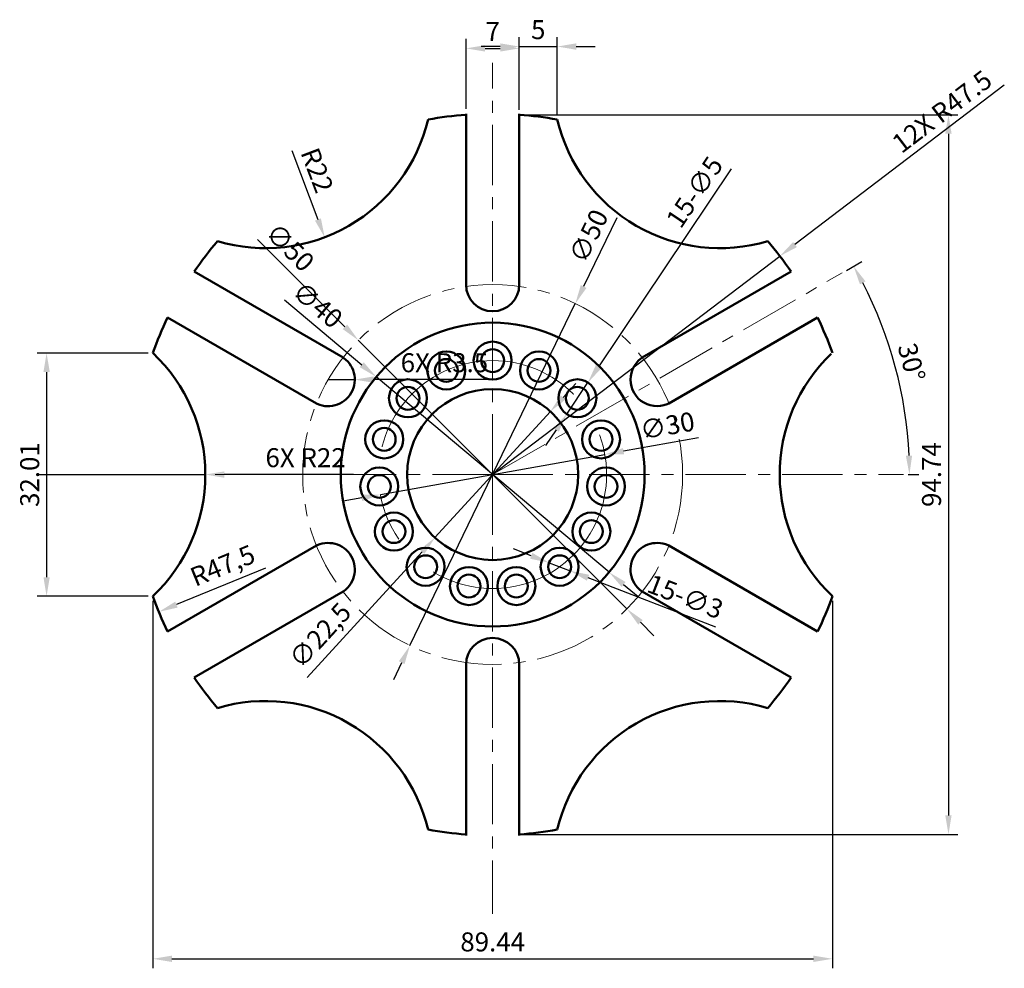
# Model space of a CAD drawing. Units: millimetres. Extents: x 3183 to 3313, y 1440 to 1565.
import ezdxf

# ---------------------------------------------------------------- set-up
doc = ezdxf.new("R2010")
doc.units = ezdxf.units.MM
doc.linetypes.add('CENTER', pattern=[50.8, 31.75, -6.35, 6.35, -6.35])
for name, color, linetype, lineweight in [('M-CNTR', 4, 'CENTER', 18), ('M-DIMS', 2, 'Continuous', 25), ('M-OUTL', 7, 'Continuous', 50)]:
    doc.layers.add(name, color=color, linetype=linetype, lineweight=lineweight)
doc.styles.get("Standard").update_dxf_attribs({"font": 'arial.ttf'})
doc.dimstyles.new('ISO-25', dxfattribs={"dimtxt": 2.5, "dimasz": 2.5, "dimexe": 1.25, "dimexo": 0.625, "dimtad": 1, "dimtxsty": 'Standard', "dimcen": 2.5, "dimadec": 0, "dimazin": 0, "dimtfac": 1, "dimtmove": 0, "dimatfit": 3, "dimfxl": 1, "dimarcsym": 0})

# ---------------------------------------------------------------- blocks, each defined once
blk = doc.blocks.new('*D1')
at = {"layer": 'Defpoints', "color": 0, "transparency": 16777216}
for p in [(3249.05, 1560.73), (3242.05, 1552.13), (3249.05, 1552.13)]:
    blk.add_point(p, dxfattribs=at)
at = {"layer": 'M-DIMS', "color": 0, "lineweight": -2, "transparency": 16777216}
for p, q in [((3242.05, 1552.75), (3242.05, 1561.98)), ((3249.05, 1552.75), (3249.05, 1561.98)), ((3244.55, 1560.73), (3246.55, 1560.73))]:
    blk.add_line(p, q, dxfattribs=at)
at = {"layer": 'M-DIMS', "color": 0, "transparency": 16777216}
for points in [[(3244.55, 1561.15), (3244.55, 1560.31), (3242.05, 1560.73)], [(3246.55, 1561.15), (3246.55, 1560.31), (3249.05, 1560.73)]]:
    blk.add_solid(points, dxfattribs=at)
at = {"layer": 'M-DIMS', "color": 0, "transparency": 16777216, "insert": (3245.55, 1562.61), "char_height": 2.5, "attachment_point": 5}
blk.add_mtext('7', dxfattribs=at)
blk = doc.blocks.new('*D2')
at = {"layer": 'Defpoints', "color": 0, "transparency": 16777216}
for p in [(3254.05, 1560.97), (3249.05, 1552), (3254.05, 1551.36)]:
    blk.add_point(p, dxfattribs=at)
at = {"layer": 'M-DIMS', "color": 0, "lineweight": -2, "transparency": 16777216}
for p, q in [((3249.05, 1552.63), (3249.05, 1562.22)), ((3254.05, 1551.99), (3254.05, 1562.22)), ((3246.55, 1560.97), (3244.05, 1560.97)), ((3249.05, 1560.97), (3254.05, 1560.97)), ((3256.55, 1560.97), (3259.05, 1560.97))]:
    blk.add_line(p, q, dxfattribs=at)
at = {"layer": 'M-DIMS', "color": 0, "transparency": 16777216}
for points in [[(3246.55, 1561.39), (3246.55, 1560.55), (3249.05, 1560.97)], [(3256.55, 1561.39), (3256.55, 1560.55), (3254.05, 1560.97)]]:
    blk.add_solid(points, dxfattribs=at)
at = {"layer": 'M-DIMS', "color": 0, "transparency": 16777216, "insert": (3251.55, 1562.87), "char_height": 2.5, "attachment_point": 5}
blk.add_mtext('5', dxfattribs=at)
blk = doc.blocks.new('*D3')
at = {"layer": 'Defpoints', "color": 0, "transparency": 16777216}
for p in [(3256.43, 1527.13), (3234.66, 1482.12)]:
    blk.add_point(p, dxfattribs=at)
at = {"layer": 'M-DIMS', "color": 0, "lineweight": -2, "transparency": 16777216}
for p, q in [((3261.9, 1538.43), (3257.52, 1529.39)), ((3234.66, 1482.12), (3256.43, 1527.13)), ((3233.57, 1479.87), (3232.48, 1477.62))]:
    blk.add_line(p, q, dxfattribs=at)
at = {"layer": 'M-DIMS', "color": 0, "transparency": 16777216}
for points in [[(3257.15, 1529.57), (3257.9, 1529.2), (3256.43, 1527.13)], [(3233.2, 1480.05), (3233.95, 1479.69), (3234.66, 1482.12)]]:
    blk.add_solid(points, dxfattribs=at)
at = {"layer": 'M-DIMS', "color": 0, "transparency": 16777216, "insert": (3258.48, 1535.89), "char_height": 2.5, "attachment_point": 5, "rotation": 64.1859}
blk.add_mtext('∅50', dxfattribs=at)
blk = doc.blocks.new('*D4')
at = {"layer": 'Defpoints', "color": 0, "transparency": 16777216}
for p in [(3258.09, 1516.74), (3255.3, 1512.59)]:
    blk.add_point(p, dxfattribs=at)
at = {"layer": 'M-DIMS', "color": 0, "lineweight": -2, "transparency": 16777216}
for p, q in [((3276.93, 1544.88), (3259.48, 1518.82)), ((3255.3, 1512.59), (3258.09, 1516.74)), ((3253.91, 1510.51), (3252.52, 1508.44))]:
    blk.add_line(p, q, dxfattribs=at)
at = {"layer": 'M-DIMS', "color": 0, "transparency": 16777216}
for points in [[(3259.13, 1519.05), (3259.82, 1518.59), (3258.09, 1516.74)], [(3253.57, 1510.74), (3254.26, 1510.28), (3255.3, 1512.59)]]:
    blk.add_solid(points, dxfattribs=at)
at = {"layer": 'M-DIMS', "color": 0, "transparency": 16777216, "insert": (3272.39, 1541.64), "char_height": 2.5, "attachment_point": 5, "rotation": 56.1832}
blk.add_mtext('15-∅5', dxfattribs=at)
blk = doc.blocks.new('*D5')
at = {"layer": 'Defpoints', "color": 0, "transparency": 16777216}
for p in [(3252.97, 1493.03), (3255.76, 1491.95)]:
    blk.add_point(p, dxfattribs=at)
at = {"layer": 'M-DIMS', "color": 0, "lineweight": -2, "transparency": 16777216}
for p, q in [((3250.63, 1493.94), (3248.3, 1494.84)), ((3252.97, 1493.03), (3255.76, 1491.95)), ((3274.94, 1484.54), (3258.1, 1491.05))]:
    blk.add_line(p, q, dxfattribs=at)
at = {"layer": 'M-DIMS', "color": 0, "transparency": 16777216}
for points in [[(3250.78, 1494.32), (3250.48, 1493.55), (3252.97, 1493.03)], [(3258.25, 1491.44), (3257.95, 1490.66), (3255.76, 1491.95)]]:
    blk.add_solid(points, dxfattribs=at)
at = {"layer": 'M-DIMS', "color": 0, "transparency": 16777216, "insert": (3270.8, 1488.26), "char_height": 2.5, "attachment_point": 5, "rotation": 338.8786}
blk.add_mtext('15-∅3', dxfattribs=at)
blk = doc.blocks.new('*D6')
at = {"layer": 'Defpoints', "color": 0, "transparency": 16777216}
for p in [(3253.14, 1512.93), (3237.96, 1496.33)]:
    blk.add_point(p, dxfattribs=at)
at = {"layer": 'M-DIMS', "color": 0, "lineweight": -2, "transparency": 16777216}
for p, q in [((3254.83, 1514.78), (3256.51, 1516.62)), ((3253.14, 1512.93), (3237.96, 1496.33)), ((3221.13, 1477.93), (3236.27, 1494.48))]:
    blk.add_line(p, q, dxfattribs=at)
at = {"layer": 'M-DIMS', "color": 0, "transparency": 16777216}
for points in [[(3254.52, 1515.06), (3255.13, 1514.5), (3253.14, 1512.93)], [(3235.96, 1494.76), (3236.58, 1494.2), (3237.96, 1496.33)]]:
    blk.add_solid(points, dxfattribs=at)
at = {"layer": 'M-DIMS', "color": 0, "transparency": 16777216, "insert": (3223.07, 1483.26), "char_height": 2.5, "attachment_point": 5, "rotation": 47.5572}
blk.add_mtext('∅22,5', dxfattribs=at)
blk = doc.blocks.new('*D7')
at = {"layer": 'Defpoints', "color": 0, "transparency": 16777216}
for p in [(3245.55, 1504.63), (3201.62, 1486.56)]:
    blk.add_point(p, dxfattribs=at)
at = {"layer": 'M-DIMS', "color": 0, "lineweight": -2, "transparency": 16777216}
blk.add_line((3215.64, 1492.32), (3203.93, 1487.51), dxfattribs=at)
at = {"layer": 'M-DIMS', "color": 0, "transparency": 16777216}
blk.add_solid([(3203.77, 1487.9), (3204.09, 1487.12), (3201.62, 1486.56)], dxfattribs=at)
at = {"layer": 'M-DIMS', "color": 0, "transparency": 16777216, "insert": (3210.13, 1492.36), "char_height": 2.5, "attachment_point": 5, "rotation": 22.3607}
blk.add_mtext('R47,5', dxfattribs=at)
blk = doc.blocks.new('*D8')
at = {"layer": 'Defpoints', "color": 0, "transparency": 16777216}
for p in [(3260.31, 1507.27), (3230.78, 1501.99)]:
    blk.add_point(p, dxfattribs=at)
at = {"layer": 'M-DIMS', "color": 0, "lineweight": -2, "transparency": 16777216}
for p, q in [((3272.66, 1509.48), (3262.77, 1507.71)), ((3230.78, 1501.99), (3260.31, 1507.27)), ((3228.32, 1501.55), (3225.86, 1501.11))]:
    blk.add_line(p, q, dxfattribs=at)
at = {"layer": 'M-DIMS', "color": 0, "transparency": 16777216}
for points in [[(3262.7, 1508.12), (3262.85, 1507.3), (3260.31, 1507.27)], [(3228.25, 1501.96), (3228.39, 1501.14), (3230.78, 1501.99)]]:
    blk.add_solid(points, dxfattribs=at)
at = {"layer": 'M-DIMS', "color": 0, "transparency": 16777216, "insert": (3268.6, 1510.75), "char_height": 2.5, "attachment_point": 5, "rotation": 10.1342}
blk.add_mtext('∅30', dxfattribs=at)
blk = doc.blocks.new('*D9')
at = {"layer": 'Defpoints', "color": 0, "transparency": 16777216}
for p in [(3291.56, 1531.19), (3299.57, 1514.15), (3245.55, 1504.63), (3245.55, 1504.63), (3299.62, 1504.63)]:
    blk.add_point(p, dxfattribs=at)
at = {"layer": 'M-DIMS', "color": 0, "lineweight": -2, "transparency": 16777216}
for p, q in [((3292.1, 1531.51), (3294.14, 1532.68)), ((3300.25, 1504.63), (3301.65, 1504.63))]:
    blk.add_line(p, q, dxfattribs=at)
blk.add_arc((3245.55, 1504.63), 54.86, 2.6114, 27.3886, dxfattribs=at)
at = {"layer": 'M-DIMS', "color": 0, "transparency": 16777216}
for points in [[(3293.89, 1529.66), (3294.62, 1530.06), (3293.05, 1532.06)], [(3300.76, 1507.14), (3299.93, 1507.12), (3300.4, 1504.63)]]:
    blk.add_solid(points, dxfattribs=at)
at = {"layer": 'M-DIMS', "color": 0, "transparency": 16777216, "insert": (3300.37, 1519.32), "char_height": 2.5, "attachment_point": 5, "rotation": 285}
blk.add_mtext('30°', dxfattribs=at)
blk = doc.blocks.new('*D10')
at = {"layer": 'Defpoints', "color": 0, "transparency": 16777216}
for p in [(3215.64, 1556.43), (3223.44, 1535.86)]:
    blk.add_point(p, dxfattribs=at)
at = {"layer": 'M-DIMS', "color": 0, "lineweight": -2, "transparency": 16777216}
blk.add_line((3219.12, 1547.27), (3222.56, 1538.2), dxfattribs=at)
at = {"layer": 'M-DIMS', "color": 0, "transparency": 16777216}
blk.add_solid([(3222.95, 1538.35), (3222.17, 1538.05), (3223.44, 1535.86)], dxfattribs=at)
at = {"layer": 'M-DIMS', "color": 0, "transparency": 16777216, "insert": (3222.15, 1544.57), "char_height": 2.5, "attachment_point": 5, "rotation": 290.7801}
blk.add_mtext('R22', dxfattribs=at)
blk = doc.blocks.new('MOUNT-HOLE-D3-D5')
for radius in [2.5, 1.5]:
    blk.add_circle((0, 0), radius)
blk = doc.blocks.new('*D12')
at = {"layer": 'Defpoints', "color": 0, "transparency": 16777216}
for p in [(3200.83, 1488.62), (3290.27, 1488.62), (3290.27, 1440.89)]:
    blk.add_point(p, dxfattribs=at)
at = {"layer": 'M-DIMS', "color": 0, "lineweight": -2, "transparency": 16777216}
for p, q in [((3200.83, 1488), (3200.83, 1439.64)), ((3290.27, 1488), (3290.27, 1439.64)), ((3203.33, 1440.89), (3287.77, 1440.89))]:
    blk.add_line(p, q, dxfattribs=at)
at = {"layer": 'M-DIMS', "color": 0, "transparency": 16777216}
for points in [[(3203.33, 1441.31), (3203.33, 1440.47), (3200.83, 1440.89)], [(3287.77, 1441.31), (3287.77, 1440.47), (3290.27, 1440.89)]]:
    blk.add_solid(points, dxfattribs=at)
at = {"layer": 'M-DIMS', "color": 0, "transparency": 16777216, "insert": (3245.55, 1442.79), "char_height": 2.5, "attachment_point": 5}
blk.add_mtext('89.44', dxfattribs=at)
blk = doc.blocks.new('*D13')
at = {"layer": 'Defpoints', "color": 0, "transparency": 16777216}
for p in [(3249.05, 1552), (3249.05, 1457.26), (3305.54, 1457.26)]:
    blk.add_point(p, dxfattribs=at)
at = {"layer": 'M-DIMS', "color": 0, "lineweight": -2, "transparency": 16777216}
for p, q in [((3249.67, 1552), (3306.79, 1552)), ((3305.54, 1549.5), (3305.54, 1459.76)), ((3249.67, 1457.26), (3306.79, 1457.26))]:
    blk.add_line(p, q, dxfattribs=at)
at = {"layer": 'M-DIMS', "color": 0, "transparency": 16777216}
for points in [[(3305.12, 1549.5), (3305.95, 1549.5), (3305.54, 1552)], [(3305.12, 1459.76), (3305.95, 1459.76), (3305.54, 1457.26)]]:
    blk.add_solid(points, dxfattribs=at)
at = {"layer": 'M-DIMS', "color": 0, "transparency": 16777216, "insert": (3303.63, 1504.63), "char_height": 2.5, "attachment_point": 5, "rotation": 90}
blk.add_mtext('94.74', dxfattribs=at)
blk = doc.blocks.new('*D14')
at = {"layer": 'Defpoints', "color": 0, "transparency": 16777216}
for p in [(3200.83, 1520.63), (3186.84, 1488.62), (3200.83, 1488.62)]:
    blk.add_point(p, dxfattribs=at)
at = {"layer": 'M-DIMS', "color": 0, "lineweight": -2, "transparency": 16777216}
for p, q in [((3200.2, 1520.63), (3185.59, 1520.63)), ((3186.84, 1518.13), (3186.84, 1491.12)), ((3200.2, 1488.62), (3185.59, 1488.62))]:
    blk.add_line(p, q, dxfattribs=at)
at = {"layer": 'M-DIMS', "color": 0, "transparency": 16777216}
for points in [[(3186.43, 1518.13), (3187.26, 1518.13), (3186.84, 1520.63)], [(3186.43, 1491.12), (3187.26, 1491.12), (3186.84, 1488.62)]]:
    blk.add_solid(points, dxfattribs=at)
at = {"layer": 'M-DIMS', "color": 0, "transparency": 16777216, "insert": (3184.94, 1504.63), "char_height": 2.5, "attachment_point": 5, "rotation": 90}
blk.add_mtext('32.01', dxfattribs=at)
blk = doc.blocks.new('*D15')
at = {"layer": 'Defpoints', "color": 0, "transparency": 16777216}
for p in [(3283.35, 1533.39), (3245.55, 1504.63)]:
    blk.add_point(p, dxfattribs=at)
at = {"layer": 'M-DIMS', "color": 0, "lineweight": -2, "transparency": 16777216}
for p, q in [((3312.89, 1555.87), (3285.34, 1534.91)), ((3245.55, 1504.63), (3283.35, 1533.39))]:
    blk.add_line(p, q, dxfattribs=at)
at = {"layer": 'M-DIMS', "color": 0, "transparency": 16777216}
blk.add_solid([(3285.09, 1535.24), (3285.59, 1534.57), (3283.35, 1533.39)], dxfattribs=at)
at = {"layer": 'M-DIMS', "color": 0, "transparency": 16777216, "insert": (3304.88, 1552.16), "char_height": 2.5, "attachment_point": 5, "rotation": 37.2672}
blk.add_mtext('12X R47.5', dxfattribs=at)
blk = doc.blocks.new('*D16')
at = {"layer": 'Defpoints', "color": 0, "transparency": 16777216}
for p in [(3185.73, 1504.63), (3207.73, 1504.63)]:
    blk.add_point(p, dxfattribs=at)
at = {"layer": 'M-DIMS', "color": 0, "lineweight": -2, "transparency": 16777216}
for p, q in [((3185.73, 1504.63), (3207.73, 1504.63)), ((3227.22, 1504.63), (3210.23, 1504.63))]:
    blk.add_line(p, q, dxfattribs=at)
at = {"layer": 'M-DIMS', "color": 0, "transparency": 16777216}
blk.add_solid([(3210.23, 1505.05), (3210.23, 1504.21), (3207.73, 1504.63)], dxfattribs=at)
at = {"layer": 'M-DIMS', "color": 0, "transparency": 16777216, "insert": (3220.93, 1506.53), "char_height": 2.5, "attachment_point": 5, "rotation": 359.999}
blk.add_mtext('6X R22', dxfattribs=at)
blk = doc.blocks.new('*D17')
at = {"layer": 'Defpoints', "color": 0, "transparency": 16777216}
for p in [(3223.9, 1517.13), (3227.4, 1517.13)]:
    blk.add_point(p, dxfattribs=at)
at = {"layer": 'M-DIMS', "color": 0, "lineweight": -2, "transparency": 16777216}
for p, q in [((3223.9, 1517.13), (3227.4, 1517.13)), ((3246, 1517.13), (3229.9, 1517.13))]:
    blk.add_line(p, q, dxfattribs=at)
at = {"layer": 'M-DIMS', "color": 0, "transparency": 16777216}
blk.add_solid([(3229.9, 1517.55), (3229.9, 1516.71), (3227.4, 1517.13)], dxfattribs=at)
at = {"layer": 'M-DIMS', "color": 0, "transparency": 16777216, "insert": (3239.2, 1519.03), "char_height": 2.5, "attachment_point": 5, "rotation": 359.9939}
blk.add_mtext('6X R3.5', dxfattribs=at)
blk = doc.blocks.new('*D18')
at = {"layer": 'Defpoints', "color": 0, "transparency": 16777216}
for p in [(3227.87, 1522.31), (3263.22, 1486.95)]:
    blk.add_point(p, dxfattribs=at)
at = {"layer": 'M-DIMS', "color": 0, "lineweight": -2, "transparency": 16777216}
for p, q in [((3214.6, 1535.58), (3226.1, 1524.08)), ((3263.22, 1486.95), (3227.87, 1522.31)), ((3264.99, 1485.18), (3266.76, 1483.41))]:
    blk.add_line(p, q, dxfattribs=at)
at = {"layer": 'M-DIMS', "color": 0, "transparency": 16777216}
for points in [[(3226.4, 1524.37), (3225.81, 1523.78), (3227.87, 1522.31)], [(3265.29, 1485.48), (3264.7, 1484.89), (3263.22, 1486.95)]]:
    blk.add_solid(points, dxfattribs=at)
at = {"layer": 'M-DIMS', "color": 0, "transparency": 16777216, "insert": (3218.66, 1534.31), "char_height": 2.5, "attachment_point": 5, "rotation": 314.9954}
blk.add_mtext('∅50', dxfattribs=at)
blk = doc.blocks.new('*D19')
at = {"layer": 'Defpoints', "color": 0, "transparency": 16777216}
for p in [(3230.23, 1517.49), (3260.87, 1491.77)]:
    blk.add_point(p, dxfattribs=at)
at = {"layer": 'M-DIMS', "color": 0, "lineweight": -2, "transparency": 16777216}
for p, q in [((3218.15, 1527.62), (3228.31, 1519.09)), ((3260.87, 1491.77), (3230.23, 1517.49)), ((3262.78, 1490.17), (3264.7, 1488.56))]:
    blk.add_line(p, q, dxfattribs=at)
at = {"layer": 'M-DIMS', "color": 0, "transparency": 16777216}
for points in [[(3228.58, 1519.41), (3228.04, 1518.77), (3230.23, 1517.49)], [(3263.05, 1490.49), (3262.52, 1489.85), (3260.87, 1491.77)]]:
    blk.add_solid(points, dxfattribs=at)
at = {"layer": 'M-DIMS', "color": 0, "transparency": 16777216, "insert": (3222.3, 1526.71), "char_height": 2.5, "attachment_point": 5, "rotation": 320.0001}
blk.add_mtext('∅40', dxfattribs=at)

msp = doc.modelspace()

# ---------------------------------------------------------------- linework, layer by layer
at = {"layer": 'M-CNTR', "ltscale": 0.25, "transparency": 33554534}
for q in [(3245.548, 1558.847), (3291.557, 1531.193), (3192.76, 1504.629), (3245.548, 1446.803), (3299.621, 1504.629)]:
    msp.add_line((3245.548, 1504.629), q, dxfattribs=at)
msp.add_circle((3245.548, 1504.629), 25, dxfattribs=at)
at = {"layer": 'M-CNTR'}
msp.add_circle((3245.548, 1504.629), 15, dxfattribs=at)
at = {"layer": 'M-OUTL'}
for p, q in [((3242.048, 1529.383), (3242.048, 1552.129)), ((3249.048, 1529.383), (3249.048, 1552.129)), ((3225.86, 1520.037), (3206.273, 1531.346)), ((3265.235, 1520.037), (3284.822, 1531.346)), ((3222.36, 1513.975), (3202.773, 1525.284)), ((3268.735, 1513.975), (3288.322, 1525.284)), ((3222.36, 1495.284), (3202.773, 1483.975)), ((3268.735, 1495.284), (3288.322, 1483.975)), ((3225.86, 1489.221), (3206.273, 1477.913)), ((3265.235, 1489.221), (3284.822, 1477.913)), ((3242.048, 1479.876), (3242.048, 1457.129)), ((3249.048, 1479.876), (3249.048, 1457.129))]:
    msp.add_line(p, q, dxfattribs=at)
for radius in [20, 11.25]:
    msp.add_circle((3245.548, 1504.629), radius, dxfattribs=at)
for centre, radius, start, end in [((3215.64, 1556.432), 22, 253.32116, 346.67885), ((3245.548, 1504.629), 47.5, 94.22562, 100.30845), ((3245.548, 1504.629), 47.5, 79.69155, 85.77438), ((3275.456, 1556.432), 22, 193.32116, 286.67884), ((3245.548, 1504.629), 47.5, 139.69155, 145.77438), ((3245.548, 1504.629), 47.5, 34.22562, 40.30845), ((3245.548, 1529.629), 3.5, 180, 0), ((3245.548, 1504.629), 47.5, 154.22562, 160.30845), ((3245.548, 1504.629), 47.5, 19.69155, 25.77438), ((3185.732, 1504.629), 22, 313.32116, 46.67884), ((3223.897, 1517.129), 3.5, 240, 60), ((3267.198, 1517.129), 3.5, 120, 300), ((3305.329, 1504.662), 22, 133.8258, 226.80251), ((3223.897, 1492.129), 3.5, 300, 120), ((3267.198, 1492.129), 3.5, 60, 240), ((3245.548, 1504.629), 47.5, 199.69155, 205.77438), ((3245.548, 1504.629), 47.5, 334.22562, 340.30845), ((3245.548, 1479.629), 3.5, 0, 180), ((3245.548, 1504.629), 47.5, 214.22562, 220.30845), ((3245.548, 1504.629), 47.5, 319.69155, 325.77438), ((3215.64, 1452.827), 22, 13.32116, 106.67884), ((3275.456, 1452.827), 22, 73.32116, 166.67884), ((3245.548, 1504.629), 47.5, 259.69155, 265.77438), ((3245.548, 1504.629), 47.5, 274.22562, 280.30845)]:
    msp.add_arc(centre, radius, start, end, dxfattribs=at)

# ---------------------------------------------------------------- block references
for p in [(3245.548, 1519.629), (3239.447, 1518.333), (3251.649, 1518.333), (3234.401, 1514.666), (3256.695, 1514.666), (3231.282, 1509.265), (3259.814, 1509.265), (3230.63, 1503.061), (3260.466, 1503.061), (3232.557, 1497.129), (3258.538, 1497.129), (3236.731, 1492.494), (3254.365, 1492.494), (3242.429, 1489.957), (3248.666, 1489.957)]:
    msp.add_blockref('MOUNT-HOLE-D3-D5', p, dxfattribs=at)

# ---------------------------------------------------------------- dimensions: what is measured, and where the dimension line sits
at = {"layer": 'M-DIMS'}
for base, p1, p2, override, picture, middle in [((3249.048, 1560.731), (3242.048, 1552.129), (3249.048, 1552.129), {"dimclrd": 0, "dimclre": 0, "dimclrt": 0}, '*D1', (3245.548, 1562.606)), ((3254.048, 1560.969), (3249.048, 1552), (3254.048, 1551.363), {"dimclrd": 0, "dimclre": 0, "dimclrt": 0}, '*D2', (3251.548, 1562.865)), ((3290.27, 1440.888), (3200.826, 1488.624), (3290.27, 1488.624), {"dimdec": 2, "dimlfac": 1, "dimrnd": 0, "dimzin": 0, "dimdsep": 46, "dimlunit": 2}, '*D12', (3245.548, 1442.79))]:
    dim = msp.add_linear_dim(base=base, p1=p1, p2=p2, dimstyle='ISO-25', override=override, dxfattribs=at)
    dim.commit()
    dim.dimension.update_dxf_attribs({"geometry": picture, "text_midpoint": middle})
for center, mpoint, text, override, picture, middle in [((3245.548, 1504.629), (3283.349, 1533.392), '12X <>', {"dimdec": 1, "dimlfac": 1, "dimrnd": 0, "dimzin": 0, "dimdsep": 46, "dimlunit": 2}, '*D15', (3306.03, 1550.65)), ((3185.732, 1504.629), (3207.732, 1504.629), '6X <>', {"dimdec": 0, "dimlfac": 1, "dimrnd": 0, "dimzin": 0, "dimdsep": 46, "dimlunit": 2}, '*D16', (3220.932, 1504.629))]:
    dim = msp.add_radius_dim(center=center, mpoint=mpoint, text=text, dimstyle='ISO-25', override=override, dxfattribs=at)
    dim.commit()
    dim.dimension.update_dxf_attribs({"geometry": picture, "text_midpoint": middle, "dimtype": 164})
for center, mpoint, picture, middle in [((3215.64, 1556.432), (3223.445, 1535.863), '*D10', (3220.394, 1543.902)), ((3245.548, 1504.629), (3201.619, 1486.559), '*D7', (3210.939, 1490.393))]:
    dim = msp.add_radius_dim(center=center, mpoint=mpoint, dimstyle='ISO-25', override={"dimclrd": 0, "dimclre": 0, "dimclrt": 0}, dxfattribs=at)
    dim.commit()
    dim.dimension.update_dxf_attribs({"geometry": picture, "text_midpoint": middle, "dimtype": 164})
for base, p1, p2, picture, middle in [((3305.536, 1457.258), (3249.048, 1552), (3249.048, 1457.258), '*D13', (3303.634, 1504.629)), ((3186.845, 1488.624), (3200.826, 1520.635), (3200.826, 1488.624), '*D14', (3184.943, 1504.629))]:
    dim = msp.add_linear_dim(base=base, p1=p1, p2=p2, angle=90, dimstyle='ISO-25', override={"dimdec": 2, "dimlfac": 1, "dimrnd": 0, "dimzin": 0, "dimdsep": 46, "dimlunit": 2}, dxfattribs=at)
    dim.commit()
    dim.dimension.update_dxf_attribs({"geometry": picture, "text_midpoint": middle})
for p1, p2, picture, middle in [((3255.304, 1512.589), (3258.086, 1516.743), '*D4', (3274.029, 1540.544)), ((3252.965, 1493.035), (3255.764, 1491.954), '*D5', (3270.085, 1486.421))]:
    dim = msp.add_diameter_dim_2p(p1=p1, p2=p2, text='15-<>', dimstyle='ISO-25', override={"dimclrd": 0, "dimclre": 0, "dimclrt": 0}, dxfattribs=at)
    dim.commit()
    dim.dimension.update_dxf_attribs({"geometry": picture, "text_midpoint": middle, "dimtype": 163})
for p1, p2, picture, middle in [((3234.661, 1482.124), (3256.434, 1527.135), '*D3', (3258.479, 1535.889)), ((3230.782, 1501.99), (3260.314, 1507.269), '*D8', (3268.601, 1510.753))]:
    dim = msp.add_diameter_dim_2p(p1=p1, p2=p2, dimstyle='ISO-25', override={"dimclrd": 0, "dimclre": 0, "dimclrt": 0}, dxfattribs=at)
    dim.commit()
    dim.dimension.update_dxf_attribs({"geometry": picture, "text_midpoint": middle})
for p1, p2, override, picture, middle in [((3263.224, 1486.95), (3227.872, 1522.308), {"dimdec": 0, "dimlfac": 1, "dimrnd": 0, "dimzin": 0, "dimdsep": 46, "dimlunit": 2}, '*D18', (3217.266, 1532.916)), ((3260.869, 1491.774), (3230.227, 1517.485), {"dimdec": 0, "dimlfac": 1, "dimrnd": 0, "dimzin": 0, "dimdsep": 46, "dimlunit": 2}, '*D19', (3221.034, 1525.199)), ((3253.14, 1512.931), (3237.956, 1496.327), {"dimclrd": 0, "dimclre": 0, "dimclrt": 0}, '*D6', (3224.672, 1481.802))]:
    dim = msp.add_diameter_dim_2p(p1=p1, p2=p2, dimstyle='ISO-25', override=override, dxfattribs=at)
    dim.commit()
    dim.dimension.update_dxf_attribs({"geometry": picture, "text_midpoint": middle, "dimtype": 163})
dim = msp.add_angular_dim_2l(base=(3299.57, 1514.155), line1=((3245.548, 1504.629), (3299.621, 1504.629)), line2=((3245.548, 1504.629), (3291.557, 1531.193)), dimstyle='ISO-25', override={"dimclrd": 0, "dimclre": 0, "dimclrt": 0}, dxfattribs=at)
dim.commit()
dim.dimension.update_dxf_attribs({"geometry": '*D9', "text_midpoint": (3300.372, 1519.319)})
dim = msp.add_radius_dim(center=(3223.897, 1517.129), mpoint=(3227.397, 1517.129), text='6X <>', dimstyle='ISO-25', override={"dimdec": 1, "dimlfac": 1, "dimrnd": 0, "dimzin": 0, "dimdsep": 46, "dimlunit": 2}, dxfattribs=at)
dim.commit()
dim.dimension.update_dxf_attribs({"geometry": '*D17', "text_midpoint": (3239.196, 1519.03)})

doc.saveas('drawing.dxf')
